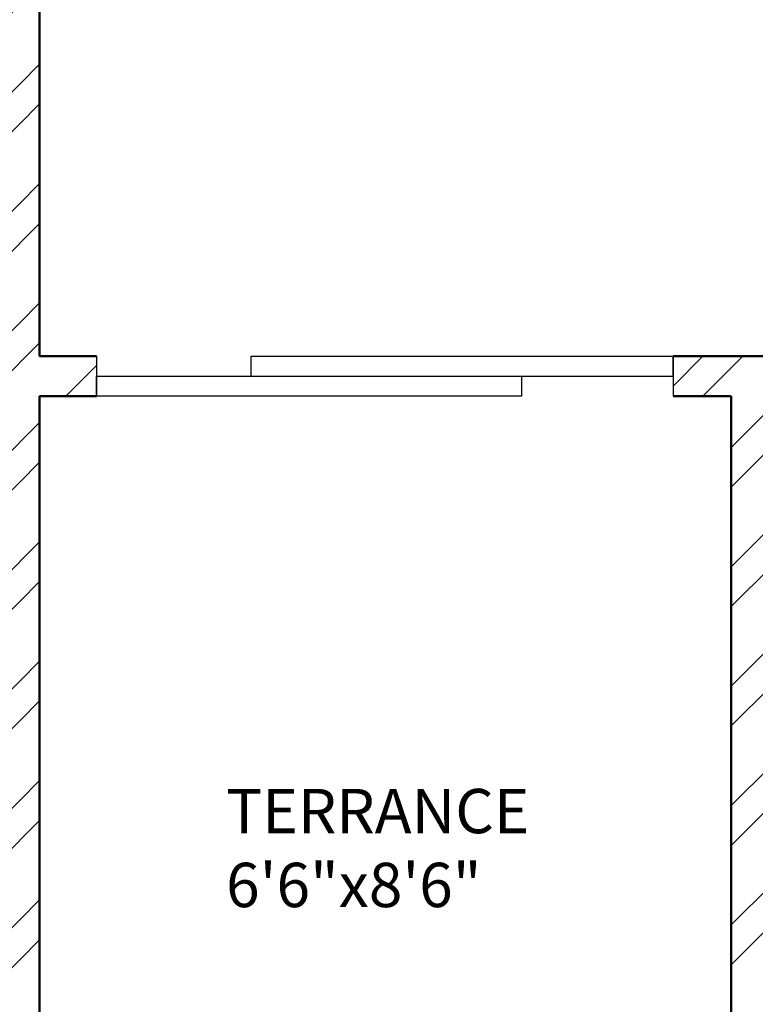
# Model space of a CAD drawing. Units: inches. Extents: x 963 to 2075, y 289 to 2657.
# Tile 31 of 98: x 1511 to 1594, y 1474 to 1585. Entities that reach past the tile are written whole.
import ezdxf

# ---------------------------------------------------------------- set-up
doc = ezdxf.new("R2010")
doc.units = ezdxf.units.IN
for name, color, linetype, lineweight in [('A-AREA-IDEN', 7, 'Continuous', 18), ('A-GLAZ', 3, 'Continuous', 25), ('A-WALL', 7, 'Continuous', 50), ('A-WALL-PATT', 8, 'Continuous', 13)]:
    doc.layers.add(name, color=color, linetype=linetype, lineweight=lineweight)
doc.styles.get("Standard").update_dxf_attribs({"font": 'arial.ttf'})

msp = doc.modelspace()

# ---------------------------------------------------------------- hatches: boundary and pattern name
at = {"layer": 'A-WALL-PATT'}
h = msp.add_hatch(dxfattribs=at)
h.set_pattern_fill('ANSI32', color=256)
h.paths.add_polyline_path([(1296.92, 2558.32), (1203.92, 2558.32), (1203.92, 2493.82), (1191.53, 2493.82), (1191.53, 2489.32), (1211.06, 2489.32), (1211.06, 2492.02), (1211.06, 2493.82), (1208.42, 2493.82), (1208.42, 2553.82), (1292.42, 2553.82), (1292.42, 2538.86), (1296.92, 2538.86)])
h.paths.add_polyline_path([(1442.42, 2558.32), (1349.42, 2558.32), (1349.42, 2538.94), (1353.92, 2538.94), (1353.92, 2553.82), (1437.92, 2553.82), (1437.92, 2493.82), (1434.54, 2493.82), (1434.54, 2489.32), (1448.31, 2489.32), (1448.31, 2491.57), (1448.31, 2493.82), (1442.42, 2493.82)])
h.paths.add_polyline_path([(1415.55, 2491.57), (1415.55, 2493.82), (1340.94, 2493.82), (1340.94, 2489.32), (1371.92, 2489.32), (1371.92, 2378.32), (1367.6, 2378.32), (1367.6, 2373.82), (1371.92, 2373.82), (1371.92, 2355.19), (1376.42, 2355.19), (1376.42, 2489.32), (1415.55, 2489.32)])
h.paths.add_polyline_path([(1304.94, 2491.57), (1304.94, 2493.82), (1296.92, 2493.82), (1296.92, 2514.86), (1292.42, 2514.86), (1292.42, 2493.82), (1232.81, 2493.82), (1232.81, 2489.32), (1256.42, 2489.32), (1256.42, 2327.32), (1253.71, 2327.32), (1253.71, 2322.82), (1328.42, 2322.82), (1328.42, 2331.15), (1323.92, 2331.15), (1323.92, 2327.32), (1260.92, 2327.32), (1260.92, 2373.82), (1323.92, 2373.82), (1323.92, 2357.81), (1328.42, 2357.81), (1328.42, 2373.82), (1346.01, 2373.82), (1346.01, 2376.07), (1346.01, 2378.32), (1260.92, 2378.32), (1260.92, 2489.32), (1304.94, 2489.32)])
h.paths.add_polyline_path([(1226.65, 2327.32), (1124.42, 2327.32), (1124.42, 2347.45), (1119.92, 2347.45), (1119.92, 2322.82), (1163.42, 2322.82), (1163.42, 2305.43), (1165.67, 2305.43), (1167.92, 2305.43), (1167.92, 2322.82), (1226.65, 2322.82), (1226.65, 2325.07)])
h.paths.add_polyline_path([(1095.92, 2489.32), (1124.42, 2489.32), (1131.53, 2489.32), (1131.53, 2491.57), (1131.53, 2493.82), (1119.92, 2493.82), (1091.42, 2493.82), (1091.42, 2417.32), (1095.92, 2417.32), (1119.92, 2417.32), (1119.92, 2407.45), (1124.42, 2407.45), (1124.42, 2421.82), (1095.92, 2421.82)])
h.paths.add_polyline_path([(1512.92, 2558.32), (1508.42, 2558.32), (1508.42, 2493.82), (1503.4, 2493.82), (1503.4, 2489.32), (1508.42, 2489.32), (1508.42, 2327.32), (1376.42, 2327.32), (1376.42, 2330.27), (1371.92, 2330.27), (1371.92, 2298.74), (1376.42, 2298.74), (1376.42, 2322.82), (1508.42, 2322.82), (1508.42, 2165.32), (1504.26, 2165.32), (1504.26, 2160.82), (1508.42, 2160.82), (1508.42, 2108.32), (1512.92, 2108.32), (1512.92, 2160.82), (1516.18, 2160.82), (1516.18, 2163.07), (1516.18, 2165.32), (1512.92, 2165.32), (1512.92, 2322.82), (1644.92, 2322.82), (1644.92, 2298.74), (1649.42, 2298.74), (1649.42, 2322.82), (1649.42, 2330.94), (1647.17, 2330.94), (1644.92, 2330.94), (1644.92, 2327.32), (1512.92, 2327.32), (1512.92, 2489.32), (1516.76, 2489.32), (1516.76, 2491.57), (1516.76, 2493.82), (1512.92, 2493.82)])
h.paths.add_polyline_path([(1671.92, 2558.32), (1578.92, 2558.32), (1578.92, 2493.82), (1573.53, 2493.82), (1573.53, 2489.32), (1586.54, 2489.32), (1586.54, 2491.57), (1586.54, 2493.82), (1583.42, 2493.82), (1583.42, 2553.82), (1667.42, 2553.82), (1667.42, 2541.11), (1671.92, 2541.11)])
h.paths.add_polyline_path([(1681.26, 2493.82), (1671.92, 2493.82), (1671.92, 2517.11), (1667.42, 2517.11), (1667.42, 2493.82), (1610.22, 2493.82), (1610.22, 2489.32), (1644.92, 2489.32), (1644.92, 2357.87), (1649.42, 2357.87), (1649.42, 2373.82), (1652.2, 2373.82), (1652.2, 2375.83), (1652.2, 2378.32), (1649.42, 2378.32), (1649.42, 2489.32), (1681.26, 2489.32), (1681.26, 2491.57)])
h.paths.add_polyline_path([(1821.92, 2558.32), (1728.92, 2558.32), (1728.92, 2541), (1733.42, 2541), (1733.42, 2553.82), (1817.42, 2553.82), (1817.42, 2493.82), (1813.51, 2493.82), (1813.51, 2489.32), (1830.08, 2489.32), (1830.08, 2491.57), (1830.08, 2493.82), (1821.92, 2493.82)])
h.paths.add_polyline_path([(1794.24, 2493.82), (1717.26, 2493.82), (1717.26, 2489.32), (1760.42, 2489.32), (1760.42, 2378.32), (1674.4, 2378.32), (1674.4, 2373.82), (1692.92, 2373.82), (1692.92, 2356.95), (1697.42, 2356.95), (1697.42, 2373.82), (1760.42, 2373.82), (1760.42, 2327.32), (1697.42, 2327.32), (1697.42, 2333.34), (1692.92, 2333.34), (1692.92, 2322.82), (1768.04, 2322.82), (1768.04, 2325.07), (1768.04, 2327.32), (1764.92, 2327.32), (1764.92, 2489.32), (1794.24, 2489.32)])
h.paths.add_polyline_path([(1733.42, 2517), (1728.92, 2517), (1728.92, 2493.82), (1733.42, 2493.82)], flags=17)
h.paths.add_polyline_path([(1929.92, 2493.82), (1890.08, 2493.82), (1890.08, 2489.32), (1896.92, 2489.32), (1925.42, 2489.32), (1925.42, 2421.82), (1896.92, 2421.82), (1896.92, 2408.32), (1901.42, 2408.32), (1901.42, 2417.32), (1925.42, 2417.32), (1929.92, 2417.32)])
h.paths.add_polyline_path([(1901.42, 2348.32), (1896.92, 2348.32), (1896.92, 2327.32), (1800.42, 2327.32), (1800.42, 2322.82), (1853.42, 2322.82), (1853.42, 2309.45), (1857.92, 2309.45), (1857.92, 2322.82), (1901.42, 2322.82)])
h.paths.add_polyline_path([(1857.92, 2249.45), (1853.42, 2249.45), (1853.42, 2214.82), (1686.31, 2214.82), (1686.31, 2210.32), (1853.42, 2210.32), (1853.42, 2202.13), (1857.92, 2202.13), (1857.92, 2210.32)])
h.paths.add_polyline_path([(1857.92, 2142.13), (1853.42, 2142.13), (1853.42, 2115.42), (1841.42, 2115.42), (1841.42, 2088.53), (1841.42, 2046.95), (1845.92, 2046.95), (1845.92, 2110.92), (1905.92, 2110.92), (1905.92, 2092.52), (1910.42, 2092.52), (1910.42, 2115.42), (1857.92, 2115.42)])
h.paths.add_polyline_path([(1532.44, 1482.34), (1573.46, 1482.34), (1573.46, 1501), (1532.44, 1501)], flags=9)
h.paths.add_polyline_path([(1438.66, 1486.3), (1479.68, 1486.3), (1479.68, 1504.96), (1438.66, 1504.96)], flags=9)
h.paths.add_polyline_path([(1411.22, 1365.31), (1659.14, 1365.31), (1659.14, 1402.4), (1411.22, 1402.4)], flags=9)
h.paths.add_polyline_path([(1185.67, 2296.3), (1248.16, 2296.3), (1248.16, 2314.95), (1185.67, 2314.95)], flags=9)
h.paths.add_polyline_path([(1177.31, 2187.35), (1216.15, 2187.35), (1216.15, 2206.01), (1177.31, 2206.01)], flags=9)
h.paths.add_polyline_path([(1295.1, 1602.08), (1328.26, 1602.08), (1328.26, 1620.74), (1295.1, 1620.74)], flags=9)
h.paths.add_polyline_path([(1525.13, 2005.99), (1558.39, 2005.99), (1558.39, 2024.65), (1525.13, 2024.65)], flags=9)
h.paths.add_polyline_path([(1459.61, 1977.13), (1472.19, 1977.13), (1472.19, 1987.43), (1459.61, 1987.43)], flags=9)
h.paths.add_polyline_path([(1467.81, 2053.68), (1480.02, 2053.68), (1480.02, 2063.98), (1467.81, 2063.98)], flags=9)
h.paths.add_polyline_path([(1555.18, 2119.02), (1584.56, 2119.02), (1584.56, 2137.68), (1555.18, 2137.68)], flags=25)
h.paths.add_polyline_path([(1405.39, 2115.29), (1444.48, 2115.29), (1444.48, 2133.95), (1405.39, 2133.95)], flags=25)
h.paths.add_polyline_path([(1698.48, 2004.26), (1727.69, 2004.26), (1727.69, 2022.92), (1698.48, 2022.92)], flags=9)
h.paths.add_polyline_path([(1612.16, 1972.86), (1629.02, 1972.86), (1629.02, 1983.16), (1612.16, 1983.16)], flags=9)
h.paths.add_polyline_path([(1608.29, 2060.04), (1625.15, 2060.04), (1625.15, 2070.34), (1608.29, 2070.34)], flags=9)
h.paths.add_polyline_path([(1527.95, 1684.4), (1566.79, 1684.4), (1566.79, 1703.06), (1527.95, 1703.06)], flags=9)
h.paths.add_polyline_path([(1422.79, 1683.59), (1461.63, 1683.59), (1461.63, 1702.25), (1422.79, 1702.25)], flags=9)
h.paths.add_polyline_path([(1531.26, 1732.46), (1574.01, 1732.46), (1574.01, 1751.12), (1531.26, 1751.12)], flags=9)
h.paths.add_polyline_path([(1402.87, 1732.85), (1439.8, 1732.85), (1439.8, 1751.5), (1402.87, 1751.5)], flags=9)
h.paths.add_polyline_path([(1243.12, 1923.13), (1281.96, 1923.13), (1281.96, 1941.79), (1243.12, 1941.79)], flags=9)
h.paths.add_polyline_path([(1181.75, 1792.27), (1244.24, 1792.27), (1244.24, 1810.93), (1181.75, 1810.93)], flags=9)
h.paths.add_polyline_path([(1265.82, 1670.3), (1316.07, 1670.3), (1316.07, 1688.96), (1265.82, 1688.96)], flags=9)
h.paths.add_polyline_path([(1140.26, 1676.05), (1179.1, 1676.05), (1179.1, 1694.71), (1140.26, 1694.71)], flags=9)
h.paths.add_polyline_path([(1107.49, 1490.89), (1143.37, 1490.89), (1143.37, 1509.55), (1107.49, 1509.55)], flags=9)
h.paths.add_polyline_path([(1217.58, 1483.9), (1246.74, 1483.9), (1246.74, 1502.56), (1217.58, 1502.56)], flags=9)
h.paths.add_polyline_path([(1389.21, 1486.92), (1418.37, 1486.92), (1418.37, 1505.58), (1389.21, 1505.58)], flags=9)
h.paths.add_polyline_path([(1672.21, 1602.08), (1705.37, 1602.08), (1705.37, 1620.74), (1672.21, 1620.74)], flags=9)
h.paths.add_polyline_path([(1752.08, 1522.64), (1781.24, 1522.64), (1781.24, 1541.3), (1752.08, 1541.3)], flags=9)
h.paths.add_polyline_path([(1848.27, 1491.26), (1884.16, 1491.26), (1884.16, 1509.92), (1848.27, 1509.92)], flags=9)
h.paths.add_polyline_path([(1822.47, 1685.62), (1861.31, 1685.62), (1861.31, 1704.28), (1822.47, 1704.28)], flags=9)
h.paths.add_polyline_path([(1713.19, 1672.23), (1763.44, 1672.23), (1763.44, 1690.89), (1713.19, 1690.89)], flags=9)
h.paths.add_polyline_path([(1736.62, 1790.58), (1799.11, 1790.58), (1799.11, 1809.24), (1736.62, 1809.24)], flags=9)
h.paths.add_polyline_path([(1691.49, 1916.36), (1730.33, 1916.36), (1730.33, 1935.01), (1691.49, 1935.01)], flags=9)
h.paths.add_polyline_path([(1764.87, 1973.92), (1794.31, 1973.92), (1794.31, 1992.58), (1764.87, 1992.58)], flags=9)
h.paths.add_polyline_path([(1767.85, 2034.02), (1797.29, 2034.02), (1797.29, 2052.67), (1767.85, 2052.67)], flags=9)
h.paths.add_polyline_path([(1851.59, 2060.33), (1880.75, 2060.33), (1880.75, 2078.99), (1851.59, 2078.99)], flags=25)
h.paths.add_polyline_path([(1688.49, 2086.87), (1727.33, 2086.87), (1727.33, 2105.53), (1688.49, 2105.53)], flags=9)
h.paths.add_polyline_path([(1537.74, 2293.58), (1580.49, 2293.58), (1580.49, 2312.24), (1537.74, 2312.24)], flags=25)
h.paths.add_polyline_path([(1425.59, 2296.11), (1468.34, 2296.11), (1468.34, 2314.77), (1425.59, 2314.77)], flags=25)
h.paths.add_polyline_path([(1278.52, 2004.18), (1307.72, 2004.18), (1307.72, 2022.84), (1278.52, 2022.84)], flags=9)
h.paths.add_polyline_path([(1193.28, 1973.63), (1222.72, 1973.63), (1222.72, 1992.29), (1193.28, 1992.29)], flags=9)
h.paths.add_polyline_path([(1192.41, 2040.58), (1221.84, 2040.58), (1221.84, 2059.23), (1192.41, 2059.23)], flags=9)
h.paths.add_polyline_path([(1130.6, 1951.39), (1159.76, 1951.39), (1159.76, 1970.05), (1130.6, 1970.05)], flags=9)
h.paths.add_polyline_path([(1132.83, 2052.49), (1161.98, 2052.49), (1161.98, 2071.15), (1132.83, 2071.15)], flags=9)
h.paths.add_polyline_path([(1265.13, 2334.62), (1315.38, 2334.62), (1315.38, 2353.28), (1265.13, 2353.28)], flags=25)
h.paths.add_polyline_path([(1136.74, 2330.79), (1175.58, 2330.79), (1175.58, 2349.44), (1136.74, 2349.44)], flags=9)
h.paths.add_polyline_path([(1287.42, 2417.2), (1320.58, 2417.2), (1320.58, 2435.86), (1287.42, 2435.86)], flags=25)
h.paths.add_polyline_path([(1430.99, 2329.16), (1469.83, 2329.16), (1469.83, 2347.82), (1430.99, 2347.82)], flags=25)
h.paths.add_polyline_path([(1525.42, 2329.21), (1564.26, 2329.21), (1564.26, 2347.87), (1525.42, 2347.87)], flags=25)
h.paths.add_polyline_path([(1684.52, 2382.8), (1717.68, 2382.8), (1717.68, 2401.46), (1684.52, 2401.46)], flags=25)
h.paths.add_polyline_path([(1704.81, 2340.29), (1755.05, 2340.29), (1755.05, 2358.95), (1704.81, 2358.95)], flags=25)
h.paths.add_polyline_path([(1694.11, 2287.76), (1756.6, 2287.76), (1756.6, 2306.41), (1694.11, 2306.41)], flags=9)
h.paths.add_polyline_path([(1815.78, 2329.86), (1854.62, 2329.86), (1854.62, 2348.52), (1815.78, 2348.52)], flags=9)
h.paths.add_polyline_path([(1842.87, 2514.26), (1878.76, 2514.26), (1878.76, 2532.91), (1842.87, 2532.91)], flags=9)
h.paths.add_polyline_path([(1769.51, 2531.45), (1798.67, 2531.45), (1798.67, 2550.1), (1769.51, 2550.1)], flags=25)
h.paths.add_polyline_path([(1594.77, 2518.47), (1623.93, 2518.47), (1623.93, 2537.13), (1594.77, 2537.13)], flags=25)
h.paths.add_polyline_path([(1520.72, 2516.18), (1556.61, 2516.18), (1556.61, 2534.84), (1520.72, 2534.84)], flags=25)
h.paths.add_polyline_path([(1464.46, 2516.69), (1500.34, 2516.69), (1500.34, 2535.35), (1464.46, 2535.35)], flags=25)
h.paths.add_polyline_path([(1365.7, 2528.97), (1394.85, 2528.97), (1394.85, 2547.63), (1365.7, 2547.63)], flags=25)
h.paths.add_polyline_path([(1222.84, 2516.23), (1252, 2516.23), (1252, 2534.89), (1222.84, 2534.89)], flags=25)
h.paths.add_polyline_path([(1104.55, 2509.6), (1140.43, 2509.6), (1140.43, 2528.26), (1104.55, 2528.26)], flags=9)
h = msp.add_hatch(dxfattribs=at)
h.set_pattern_fill('ANSI32', color=256)
h.paths.add_polyline_path([(1335.97, 2212.57), (1335.97, 2214.82), (1167.92, 2214.82), (1167.92, 2245.43), (1163.42, 2245.43), (1163.42, 2210.32), (1163.42, 2194.81), (1167.92, 2194.81), (1167.92, 2210.32), (1335.97, 2210.32)])
h.paths.add_polyline_path([(1532.44, 1482.34), (1573.46, 1482.34), (1573.46, 1501), (1532.44, 1501)], flags=9)
h.paths.add_polyline_path([(1438.66, 1486.3), (1479.68, 1486.3), (1479.68, 1504.96), (1438.66, 1504.96)], flags=9)
h.paths.add_polyline_path([(1411.22, 1365.31), (1659.14, 1365.31), (1659.14, 1402.4), (1411.22, 1402.4)], flags=9)
h.paths.add_polyline_path([(1185.67, 2296.3), (1248.16, 2296.3), (1248.16, 2314.95), (1185.67, 2314.95)], flags=9)
h.paths.add_polyline_path([(1177.31, 2187.35), (1216.15, 2187.35), (1216.15, 2206.01), (1177.31, 2206.01)], flags=9)
h.paths.add_polyline_path([(1295.1, 1602.08), (1328.26, 1602.08), (1328.26, 1620.74), (1295.1, 1620.74)], flags=9)
h.paths.add_polyline_path([(1525.13, 2005.99), (1558.39, 2005.99), (1558.39, 2024.65), (1525.13, 2024.65)], flags=9)
h.paths.add_polyline_path([(1459.61, 1977.13), (1472.19, 1977.13), (1472.19, 1987.43), (1459.61, 1987.43)], flags=9)
h.paths.add_polyline_path([(1467.81, 2053.68), (1480.02, 2053.68), (1480.02, 2063.98), (1467.81, 2063.98)], flags=9)
h.paths.add_polyline_path([(1555.18, 2119.02), (1584.56, 2119.02), (1584.56, 2137.68), (1555.18, 2137.68)], flags=9)
h.paths.add_polyline_path([(1405.39, 2115.29), (1444.48, 2115.29), (1444.48, 2133.95), (1405.39, 2133.95)], flags=9)
h.paths.add_polyline_path([(1698.48, 2004.26), (1727.69, 2004.26), (1727.69, 2022.92), (1698.48, 2022.92)], flags=9)
h.paths.add_polyline_path([(1612.16, 1972.86), (1629.02, 1972.86), (1629.02, 1983.16), (1612.16, 1983.16)], flags=9)
h.paths.add_polyline_path([(1608.29, 2060.04), (1625.15, 2060.04), (1625.15, 2070.34), (1608.29, 2070.34)], flags=9)
h.paths.add_polyline_path([(1527.95, 1684.4), (1566.79, 1684.4), (1566.79, 1703.06), (1527.95, 1703.06)], flags=9)
h.paths.add_polyline_path([(1422.79, 1683.59), (1461.63, 1683.59), (1461.63, 1702.25), (1422.79, 1702.25)], flags=9)
h.paths.add_polyline_path([(1531.26, 1732.46), (1574.01, 1732.46), (1574.01, 1751.12), (1531.26, 1751.12)], flags=9)
h.paths.add_polyline_path([(1402.87, 1732.85), (1439.8, 1732.85), (1439.8, 1751.5), (1402.87, 1751.5)], flags=9)
h.paths.add_polyline_path([(1243.12, 1923.13), (1281.96, 1923.13), (1281.96, 1941.79), (1243.12, 1941.79)], flags=9)
h.paths.add_polyline_path([(1181.75, 1792.27), (1244.24, 1792.27), (1244.24, 1810.93), (1181.75, 1810.93)], flags=9)
h.paths.add_polyline_path([(1265.82, 1670.3), (1316.07, 1670.3), (1316.07, 1688.96), (1265.82, 1688.96)], flags=9)
h.paths.add_polyline_path([(1140.26, 1676.05), (1179.1, 1676.05), (1179.1, 1694.71), (1140.26, 1694.71)], flags=9)
h.paths.add_polyline_path([(1107.49, 1490.89), (1143.37, 1490.89), (1143.37, 1509.55), (1107.49, 1509.55)], flags=9)
h.paths.add_polyline_path([(1217.58, 1483.9), (1246.74, 1483.9), (1246.74, 1502.56), (1217.58, 1502.56)], flags=9)
h.paths.add_polyline_path([(1389.21, 1486.92), (1418.37, 1486.92), (1418.37, 1505.58), (1389.21, 1505.58)], flags=9)
h.paths.add_polyline_path([(1672.21, 1602.08), (1705.37, 1602.08), (1705.37, 1620.74), (1672.21, 1620.74)], flags=9)
h.paths.add_polyline_path([(1752.08, 1522.64), (1781.24, 1522.64), (1781.24, 1541.3), (1752.08, 1541.3)], flags=9)
h.paths.add_polyline_path([(1848.27, 1491.26), (1884.16, 1491.26), (1884.16, 1509.92), (1848.27, 1509.92)], flags=9)
h.paths.add_polyline_path([(1822.47, 1685.62), (1861.31, 1685.62), (1861.31, 1704.28), (1822.47, 1704.28)], flags=9)
h.paths.add_polyline_path([(1713.19, 1672.23), (1763.44, 1672.23), (1763.44, 1690.89), (1713.19, 1690.89)], flags=9)
h.paths.add_polyline_path([(1736.62, 1790.58), (1799.11, 1790.58), (1799.11, 1809.24), (1736.62, 1809.24)], flags=9)
h.paths.add_polyline_path([(1691.49, 1916.36), (1730.33, 1916.36), (1730.33, 1935.01), (1691.49, 1935.01)], flags=9)
h.paths.add_polyline_path([(1764.87, 1973.92), (1794.31, 1973.92), (1794.31, 1992.58), (1764.87, 1992.58)], flags=9)
h.paths.add_polyline_path([(1767.85, 2034.02), (1797.29, 2034.02), (1797.29, 2052.67), (1767.85, 2052.67)], flags=9)
h.paths.add_polyline_path([(1851.59, 2060.33), (1880.75, 2060.33), (1880.75, 2078.99), (1851.59, 2078.99)], flags=9)
h.paths.add_polyline_path([(1688.49, 2086.87), (1727.33, 2086.87), (1727.33, 2105.53), (1688.49, 2105.53)], flags=9)
h.paths.add_polyline_path([(1537.74, 2293.58), (1580.49, 2293.58), (1580.49, 2312.24), (1537.74, 2312.24)], flags=9)
h.paths.add_polyline_path([(1425.59, 2296.11), (1468.34, 2296.11), (1468.34, 2314.77), (1425.59, 2314.77)], flags=9)
h.paths.add_polyline_path([(1278.52, 2004.18), (1307.72, 2004.18), (1307.72, 2022.84), (1278.52, 2022.84)], flags=9)
h.paths.add_polyline_path([(1193.28, 1973.63), (1222.72, 1973.63), (1222.72, 1992.29), (1193.28, 1992.29)], flags=9)
h.paths.add_polyline_path([(1192.41, 2040.58), (1221.84, 2040.58), (1221.84, 2059.23), (1192.41, 2059.23)], flags=9)
h.paths.add_polyline_path([(1130.6, 1951.39), (1159.76, 1951.39), (1159.76, 1970.05), (1130.6, 1970.05)], flags=9)
h.paths.add_polyline_path([(1132.83, 2052.49), (1161.98, 2052.49), (1161.98, 2071.15), (1132.83, 2071.15)], flags=9)
h.paths.add_polyline_path([(1265.13, 2334.62), (1315.38, 2334.62), (1315.38, 2353.28), (1265.13, 2353.28)], flags=9)
h.paths.add_polyline_path([(1136.74, 2330.79), (1175.58, 2330.79), (1175.58, 2349.44), (1136.74, 2349.44)], flags=9)
h.paths.add_polyline_path([(1287.42, 2417.2), (1320.58, 2417.2), (1320.58, 2435.86), (1287.42, 2435.86)], flags=9)
h.paths.add_polyline_path([(1430.99, 2329.16), (1469.83, 2329.16), (1469.83, 2347.82), (1430.99, 2347.82)], flags=9)
h.paths.add_polyline_path([(1525.42, 2329.21), (1564.26, 2329.21), (1564.26, 2347.87), (1525.42, 2347.87)], flags=9)
h.paths.add_polyline_path([(1684.52, 2382.8), (1717.68, 2382.8), (1717.68, 2401.46), (1684.52, 2401.46)], flags=9)
h.paths.add_polyline_path([(1704.81, 2340.29), (1755.05, 2340.29), (1755.05, 2358.95), (1704.81, 2358.95)], flags=9)
h.paths.add_polyline_path([(1694.11, 2287.76), (1756.6, 2287.76), (1756.6, 2306.41), (1694.11, 2306.41)], flags=9)
h.paths.add_polyline_path([(1815.78, 2329.86), (1854.62, 2329.86), (1854.62, 2348.52), (1815.78, 2348.52)], flags=9)
h.paths.add_polyline_path([(1842.87, 2514.26), (1878.76, 2514.26), (1878.76, 2532.91), (1842.87, 2532.91)], flags=9)
h.paths.add_polyline_path([(1769.51, 2531.45), (1798.67, 2531.45), (1798.67, 2550.1), (1769.51, 2550.1)], flags=9)
h.paths.add_polyline_path([(1594.77, 2518.47), (1623.93, 2518.47), (1623.93, 2537.13), (1594.77, 2537.13)], flags=9)
h.paths.add_polyline_path([(1520.72, 2516.18), (1556.61, 2516.18), (1556.61, 2534.84), (1520.72, 2534.84)], flags=9)
h.paths.add_polyline_path([(1464.46, 2516.69), (1500.34, 2516.69), (1500.34, 2535.35), (1464.46, 2535.35)], flags=9)
h.paths.add_polyline_path([(1365.7, 2528.97), (1394.85, 2528.97), (1394.85, 2547.63), (1365.7, 2547.63)], flags=9)
h.paths.add_polyline_path([(1222.84, 2516.23), (1252, 2516.23), (1252, 2534.89), (1222.84, 2534.89)], flags=9)
h.paths.add_polyline_path([(1104.55, 2509.6), (1140.43, 2509.6), (1140.43, 2528.26), (1104.55, 2528.26)], flags=9)
h = msp.add_hatch(dxfattribs=at)
h.set_pattern_fill('ANSI32', color=256)
h.paths.add_polyline_path([(1473.61, 2163.07), (1473.61, 2165.32), (1376.42, 2165.32), (1376.42, 2227.98), (1371.92, 2227.98), (1371.92, 2214.82), (1368.41, 2214.82), (1368.41, 2210.32), (1371.92, 2210.32), (1371.92, 2160.82), (1395.92, 2160.82), (1395.92, 2090.32), (1217.34, 2090.32), (1217.34, 2085.82), (1395.92, 2085.82), (1458.92, 2085.82), (1458.92, 2108.32), (1454.42, 2108.32), (1454.42, 2090.32), (1400.42, 2090.32), (1400.42, 2160.82), (1473.61, 2160.82)])
h.paths.add_polyline_path([(1649.42, 2210.32), (1653.23, 2210.32), (1653.23, 2214.82), (1649.42, 2214.82), (1649.42, 2227.98), (1644.92, 2227.98), (1644.92, 2165.32), (1550.1, 2165.32), (1550.1, 2160.82), (1620.92, 2160.82), (1620.92, 2112.82), (1555.45, 2112.82), (1555.45, 2108.32), (1584.33, 2108.32), (1584.33, 2084.92), (1588.83, 2084.92), (1588.83, 2108.32), (1625.42, 2108.32), (1667.95, 2108.32), (1667.95, 2022.67), (1588.83, 2022.67), (1588.83, 2047.41), (1584.33, 2047.41), (1584.33, 1996), (1588.83, 1996), (1588.83, 2018.32), (1667.95, 2018.17), (1667.95, 1928.32), (1625.42, 1928.32), (1625.42, 1923.82), (1672.45, 1923.82), (1672.45, 1928.32), (1672.45, 1946.66), (1785.45, 1946.66), (1785.45, 1951.16), (1743.03, 1951.16), (1743.03, 2017.92), (1841.42, 2017.92), (1841.42, 2014.77), (1845.92, 2014.77), (1845.92, 2017.92), (1905.92, 2017.92), (1905.92, 1987.51), (1910.42, 1987.51), (1910.42, 2022.42), (1910.42, 2068.52), (1905.92, 2068.52), (1905.92, 2022.42), (1845.92, 2022.42), (1845.92, 2025.85), (1843.67, 2025.85), (1841.42, 2025.85), (1841.42, 2022.42), (1743.03, 2022.42), (1743.03, 2084.03), (1768.45, 2084.03), (1785.45, 2084.03), (1785.45, 2088.53), (1672.45, 2088.53), (1672.45, 2112.82), (1667.95, 2112.82), (1625.42, 2112.82), (1625.42, 2160.82), (1649.42, 2160.82)])
h.paths.add_polyline_path([(1672.45, 2084.03), (1738.53, 2084.03), (1738.53, 1951.16), (1672.45, 1951.16)], flags=16)
h.paths.add_polyline_path([(1672.45, 2084.03), (1738.53, 2084.03), (1705.49, 2017.6)], flags=0)
h.paths.add_polyline_path([(1262.77, 2085.82), (1258.27, 2085.82), (1258.27, 2023.28), (1184.42, 2023.28), (1184.42, 2018.78), (1258.27, 2018.78), (1258.27, 1950.82), (1262.77, 1950.82)])
h.paths.add_polyline_path([(1312.27, 2085.82), (1307.77, 2085.82), (1307.77, 1950.82), (1312.27, 1950.82)])
h.paths.add_polyline_path([(1458.92, 1950.82), (1395.92, 1950.82), (1216.57, 1950.82), (1216.57, 1946.32), (1346.42, 1946.32), (1395.92, 1946.32), (1395.92, 1875.82), (1371.92, 1875.82), (1371.92, 1826.32), (1368.93, 1826.32), (1368.93, 1821.82), (1371.92, 1821.82), (1371.92, 1813.62), (1376.42, 1813.62), (1376.42, 1871.32), (1474.5, 1871.32), (1474.5, 1873.57), (1474.5, 1875.82), (1400.42, 1875.82), (1400.42, 1946.32), (1454.42, 1946.32), (1454.42, 1928.32), (1458.92, 1928.32)])
h.paths.add_polyline_path([(1184.42, 2120.78), (1167.92, 2120.78), (1167.92, 2134.81), (1165.67, 2134.81), (1163.42, 2134.81), (1163.42, 2120.78), (1119.92, 2120.78), (1119.92, 2098.1), (1124.42, 2098.1), (1124.42, 2116.28), (1167.92, 2116.28), (1179.92, 2116.28), (1179.92, 2045.92), (1184.42, 2045.92), (1184.42, 2090.32), (1184.42, 2116.28)])
h.paths.add_polyline_path([(1124.42, 2018.78), (1179.92, 2018.78), (1179.92, 2016.29), (1184.42, 2016.29), (1184.42, 2023.28), (1184.42, 2026.59), (1182.17, 2026.59), (1179.92, 2026.59), (1179.92, 2023.28), (1124.42, 2023.28), (1124.42, 2074.1), (1119.92, 2074.1), (1119.92, 2018.78), (1119.92, 1979.63), (1124.42, 1979.63)])
h.paths.add_polyline_path([(1184.42, 1925.78), (1184.42, 1946.32), (1184.42, 1996.07), (1182.17, 1996.07), (1179.92, 1996.07), (1179.92, 1925.78), (1124.42, 1925.78), (1124.42, 1955.63), (1119.92, 1955.5), (1119.92, 1921.28), (1158.92, 1921.28), (1158.92, 1909.98), (1163.42, 1909.98), (1163.42, 1921.28), (1184.42, 1921.28)])
h.paths.add_polyline_path([(1341.45, 1826.32), (1163.42, 1826.32), (1163.42, 1849.98), (1158.92, 1849.98), (1158.92, 1821.82), (1158.92, 1804.03), (1163.42, 1804.03), (1163.42, 1821.82), (1341.45, 1821.82)])
h.paths.add_polyline_path([(1222.98, 1713.82), (1163.42, 1713.82), (1163.42, 1744.03), (1161.17, 1744.03), (1158.92, 1744.03), (1158.92, 1713.82), (1119.92, 1713.82), (1119.92, 1694.65), (1124.42, 1694.65), (1124.42, 1709.32), (1158.92, 1709.32), (1222.98, 1709.32)])
h.paths.add_polyline_path([(1328.42, 1713.82), (1252.04, 1713.82), (1252.04, 1711.57), (1252.04, 1709.32), (1256.42, 1709.32), (1256.42, 1547.32), (1232.94, 1547.32), (1232.94, 1545.07), (1232.94, 1542.82), (1292.42, 1542.82), (1292.42, 1527.63), (1296.92, 1527.63), (1296.92, 1542.82), (1299.46, 1542.82), (1299.46, 1547.32), (1260.92, 1547.32), (1260.92, 1658.32), (1343.66, 1658.32), (1343.66, 1660.57), (1343.66, 1662.82), (1328.42, 1662.82), (1328.42, 1676.59), (1327.4, 1676.59), (1323.92, 1676.59), (1323.92, 1662.82), (1260.92, 1662.82), (1260.92, 1709.32), (1323.92, 1709.32), (1323.92, 1699.85), (1328.42, 1699.85)])
h.paths.add_polyline_path([(1649.42, 1875.82), (1625.42, 1875.82), (1625.42, 1928.32), (1620.92, 1928.32), (1588.83, 1928.32), (1588.83, 1950.59), (1584.33, 1950.59), (1584.33, 1928.32), (1555.45, 1928.32), (1555.45, 1923.82), (1620.92, 1923.82), (1620.92, 1875.82), (1548.95, 1875.82), (1548.95, 1873.57), (1548.95, 1871.32), (1644.92, 1871.32), (1644.92, 1813.62), (1649.42, 1813.62), (1649.42, 1821.82), (1652.04, 1821.82), (1652.04, 1824.07), (1652.04, 1826.32), (1649.42, 1826.32)])
h.paths.add_polyline_path([(1512.92, 1871.32), (1516.48, 1871.32), (1516.48, 1875.82), (1512.92, 1875.82), (1512.92, 1923.82), (1512.92, 1928.32), (1512.92, 1930.83), (1508.42, 1930.83), (1508.42, 1875.82), (1504.41, 1875.82), (1504.41, 1871.32), (1508.42, 1871.32), (1508.42, 1713.82), (1376.42, 1713.82), (1376.42, 1743.32), (1371.92, 1743.32), (1371.92, 1709.32), (1371.92, 1706.01), (1376.42, 1706.01), (1376.42, 1709.32), (1508.42, 1709.32), (1508.42, 1547.32), (1501.87, 1547.32), (1501.87, 1542.82), (1508.42, 1542.82), (1508.42, 1482.82), (1508.42, 1436.32), (1512.92, 1436.32), (1512.92, 1542.82), (1519.32, 1542.82), (1519.32, 1545.07), (1519.32, 1547.32), (1512.92, 1547.32), (1512.92, 1709.32), (1644.92, 1709.32), (1644.92, 1707.55), (1649.42, 1707.55), (1649.42, 1709.32), (1649.42, 1743.32), (1644.92, 1743.32), (1644.92, 1713.82), (1512.92, 1713.82)])
h.paths.add_polyline_path([(1129.88, 1545.07), (1129.88, 1547.32), (1124.42, 1547.32), (1095.92, 1547.32), (1095.92, 1614.82), (1124.42, 1614.82), (1124.42, 1619.32), (1095.92, 1619.32), (1091.42, 1619.32), (1091.42, 1542.82), (1095.92, 1542.82), (1119.92, 1542.82), (1129.88, 1542.82)])
h.paths.add_polyline_path([(1208.42, 1542.82), (1211.74, 1542.82), (1211.74, 1547.32), (1198.85, 1547.32), (1198.85, 1542.82), (1203.92, 1542.82), (1203.92, 1478.32), (1208.42, 1478.32), (1296.92, 1478.32), (1296.92, 1503.63), (1292.42, 1503.63), (1292.42, 1482.82), (1208.42, 1482.82)])
h.paths.add_polyline_path([(1430.42, 1542.82), (1435.7, 1542.82), (1435.7, 1545.07), (1435.7, 1547.32), (1422.66, 1547.32), (1422.66, 1545.07), (1422.66, 1542.82), (1425.92, 1542.82), (1425.92, 1482.86), (1341.92, 1482.86), (1341.92, 1502.73), (1337.42, 1502.73), (1337.42, 1478.36), (1425.92, 1478.36), (1425.92, 1440.82), (1425.92, 1436.32), (1430.42, 1436.32)])
h.paths.add_polyline_path([(1698.48, 2004.26), (1727.69, 2004.26), (1727.69, 2022.92), (1698.48, 2022.92)], flags=8)
h = msp.add_hatch(dxfattribs=at)
h.set_pattern_fill('ANSI32', color=256)
h.paths.add_polyline_path([(1910.42, 1929.42), (1910.42, 1963.51), (1905.92, 1963.51), (1905.92, 1929.42), (1845.92, 1929.42), (1845.92, 1993.37), (1843.67, 1993.37), (1841.42, 1993.37), (1841.42, 1951.16), (1841.42, 1924.92), (1853.42, 1924.92), (1853.42, 1913.07), (1857.92, 1913.07), (1857.92, 1924.92), (1910.42, 1924.92)])
h.paths.add_polyline_path([(1857.92, 1853.07), (1853.42, 1853.07), (1853.42, 1826.32), (1841.42, 1826.32), (1674.48, 1826.32), (1674.48, 1821.82), (1853.42, 1821.82), (1857.92, 1821.82)])
h.paths.add_polyline_path([(1857.92, 1821.82), (1853.42, 1821.82), (1853.42, 1807.79), (1857.92, 1807.79)])
h.paths.add_polyline_path([(1857.92, 1747.79), (1853.42, 1747.79), (1853.42, 1713.82), (1809.34, 1713.82), (1809.34, 1709.32), (1905.92, 1709.32), (1905.92, 1688.32), (1910.42, 1688.32), (1910.42, 1713.82), (1857.92, 1713.82)])
h.paths.add_polyline_path([(1830.92, 1542.82), (1837.43, 1542.82), (1837.43, 1545.07), (1837.43, 1547.32), (1823.42, 1547.32), (1823.42, 1545.07), (1823.42, 1542.82), (1826.42, 1542.82), (1826.42, 1482.82), (1742.42, 1482.82), (1742.42, 1505.39), (1737.92, 1505.39), (1737.92, 1478.32), (1830.92, 1478.32)])
h.paths.add_polyline_path([(1938.92, 1619.32), (1934.42, 1619.32), (1910.42, 1619.32), (1910.42, 1628.32), (1908.17, 1628.32), (1905.92, 1628.32), (1905.92, 1614.82), (1934.42, 1614.82), (1934.42, 1547.32), (1905.92, 1547.32), (1899.59, 1547.32), (1899.59, 1542.82), (1910.42, 1542.82), (1938.92, 1542.82)])
h.paths.add_polyline_path([(1803.68, 1547.32), (1773.92, 1547.32), (1773.92, 1709.32), (1777.76, 1709.32), (1777.76, 1713.82), (1701.92, 1713.82), (1701.92, 1697.8), (1706.42, 1697.8), (1706.42, 1709.32), (1769.42, 1709.32), (1769.42, 1662.82), (1706.42, 1662.82), (1706.42, 1674.38), (1701.92, 1674.38), (1701.92, 1662.82), (1675.67, 1662.82), (1675.67, 1658.32), (1769.42, 1658.32), (1769.42, 1547.32), (1729.17, 1547.32), (1729.17, 1542.82), (1737.92, 1542.82), (1737.92, 1529.39), (1742.42, 1529.39), (1742.42, 1542.82), (1803.68, 1542.82)])
h.paths.add_polyline_path([(1595.42, 1542.82), (1599.24, 1542.82), (1599.24, 1547.32), (1584.36, 1547.32), (1584.36, 1542.82), (1590.92, 1542.82), (1590.92, 1436.32), (1595.42, 1436.32), (1595.42, 1440.82)])
h.paths.add_polyline_path([(1693.17, 1547.32), (1649.42, 1547.32), (1649.42, 1658.32), (1652.1, 1658.32), (1652.1, 1660.57), (1652.1, 1662.82), (1649.42, 1662.82), (1649.42, 1680.94), (1647.17, 1680.94), (1644.92, 1680.94), (1644.92, 1547.32), (1622.42, 1547.32), (1622.42, 1545.07), (1622.42, 1542.82), (1649.42, 1542.82), (1679.42, 1542.82), (1679.42, 1529.85), (1681.67, 1529.85), (1683.92, 1529.85), (1683.92, 1542.82), (1693.17, 1542.82), (1693.17, 1545.07)])
h.paths.add_polyline_path([(1683.92, 1505.85), (1679.42, 1505.85), (1679.42, 1483.8), (1595.42, 1483.8), (1595.42, 1479.3), (1683.92, 1479.3)])
h.paths.add_polyline_path([(1402.99, 1547.32), (1376.42, 1547.32), (1376.42, 1675.89), (1374.17, 1675.89), (1371.92, 1675.89), (1371.92, 1662.82), (1368.88, 1662.82), (1368.88, 1658.32), (1371.92, 1658.32), (1371.92, 1547.32), (1335.46, 1547.32), (1335.46, 1542.82), (1337.42, 1542.82), (1337.42, 1526.73), (1341.92, 1526.73), (1341.92, 1542.82), (1371.92, 1542.82), (1402.99, 1542.82)])

# ---------------------------------------------------------------- linework, layer by layer
at = {"layer": 'A-GLAZ'}
for p, q in [((1519.32, 1547.32), (1519.32, 1542.82)), ((1536.78, 1547.32), (1584.36, 1547.32)), ((1536.78, 1545.07), (1536.78, 1547.32)), ((1584.36, 1545.07), (1584.36, 1547.32)), ((1584.36, 1547.32), (1584.36, 1542.82)), ((1519.32, 1542.82), (1519.32, 1545.07)), ((1519.32, 1545.07), (1582.96, 1545.07)), ((1567.25, 1545.07), (1567.25, 1542.82)), ((1582.96, 1545.07), (1584.36, 1545.07)), ((1567.25, 1542.82), (1519.32, 1542.82))]:
    msp.add_line(p, q, dxfattribs=at)
at = {"layer": 'A-WALL'}
for p, q in [((1512.92, 1547.32), (1512.92, 1709.32)), ((1519.32, 1547.32), (1512.92, 1547.32)), ((1599.24, 1547.32), (1584.36, 1547.32)), ((1512.92, 1542.82), (1512.92, 1436.32)), ((1519.32, 1542.82), (1512.92, 1542.82)), ((1590.92, 1542.82), (1584.36, 1542.82)), ((1590.92, 1436.32), (1590.92, 1542.82))]:
    msp.add_line(p, q, dxfattribs=at)

# ---------------------------------------------------------------- texts
at = {"layer": 'A-AREA-IDEN', "insert": (1533.95, 1498.51), "char_height": 5, "attachment_point": 1}
msp.add_mtext_dynamic_manual_height_columns('TERRANCE\\P6\'6"x8\'6"', width=108.2314, gutter_width=12.5, heights=[0], dxfattribs=at)

doc.saveas('drawing.dxf')
